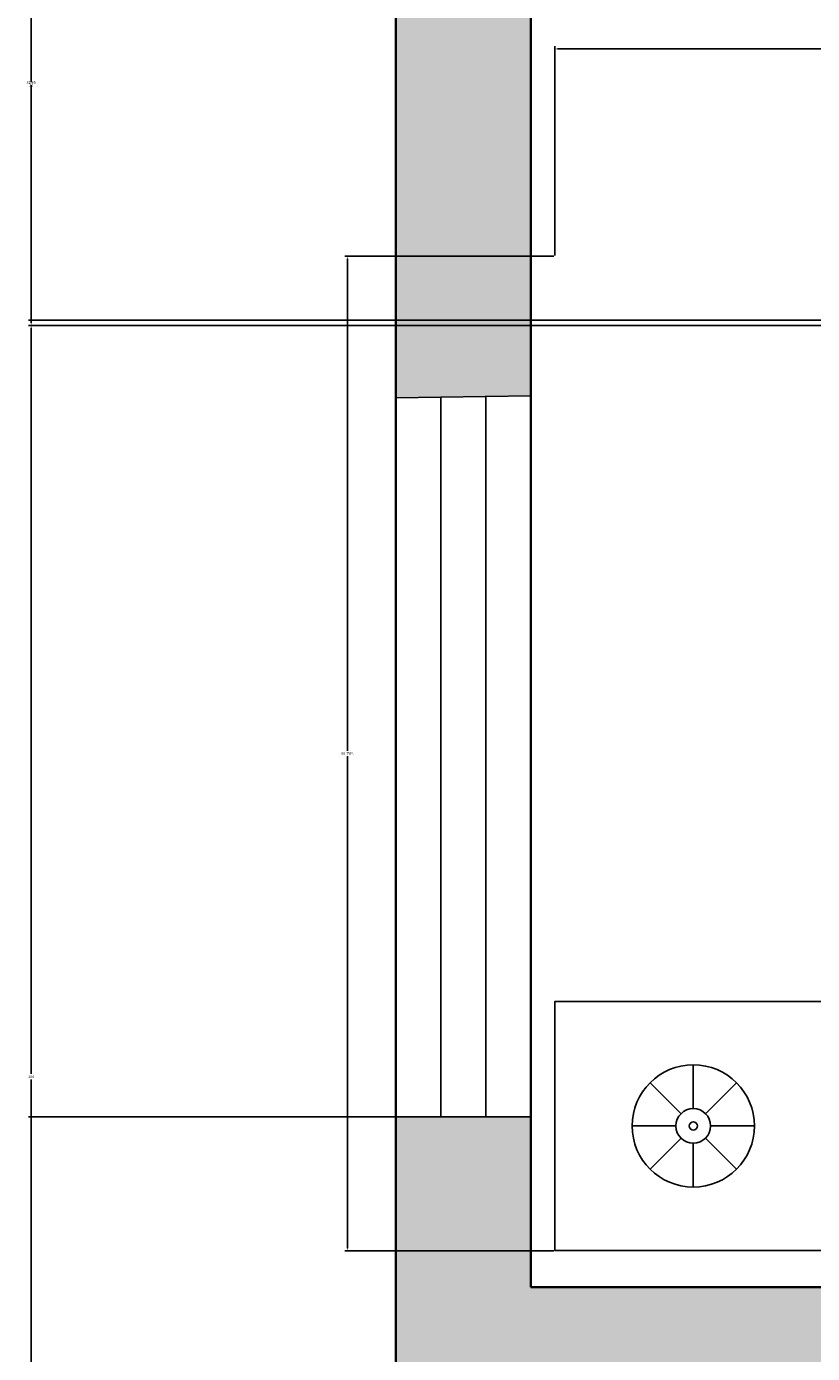
# Model space of a CAD drawing. Units: millimetres. Extents: x 2817 to 5038, y 1110 to 3565.
# Tile 11 of 21: x 2817 to 2869, y 1505 to 1593. Entities that reach past the tile are written whole.
import ezdxf

# ---------------------------------------------------------------- set-up
doc = ezdxf.new("R2010")
doc.units = ezdxf.units.MM
for name, color, linetype, lineweight in [('A-ANNO-DIMS', 2, 'Continuous', 18), ('A-WALL', 7, 'Continuous', 35), ('DOOR&WINDOW', 1, 'Continuous', 25), ('FURNITURE', 219, 'Continuous', 18)]:
    doc.layers.add(name, color=color, linetype=linetype, lineweight=lineweight)
doc.layers.add('A-WALL-PATT', color=51, linetype='Continuous', lineweight=13, true_color=0xf7f281)
doc.layers.add('BLOCK', color=6, linetype='Continuous')
doc.styles.get("Standard").update_dxf_attribs({"font": 'arial.ttf'})
doc.dimstyles.get("Standard").update_dxf_attribs({"dimtxt": 0.18, "dimasz": 0.18, "dimexe": 0.18, "dimexo": 0.0625, "dimgap": 0.09, "dimtad": 0, "dimtih": 1, "dimtoh": 1, "dimdec": 4, "dimzin": 0, "dimdsep": 46, "dimtxsty": 'Standard', "dimcen": 0.09, "dimadec": 0, "dimazin": 0, "dimtfac": 1, "dimtdec": 4, "dimtofl": 0, "dimtmove": 0, "dimatfit": 3, "dimfxl": 1, "dimtolj": 1, "dimtzin": 0, "dimarcsym": 0})

# ---------------------------------------------------------------- blocks, each defined once
blk = doc.blocks.new('A$C52E67D0D')
at = {"layer": 'BLOCK'}
for p, q in [((2251.5, 1605.5), (2251.5, 1684.7)), ((2229.3, 1596.3), (2173.3, 1652.3)), ((2273.7, 1596.3), (2329.7, 1652.3)), ((2220.1, 1574.1), (2140.9, 1574.1)), ((2282.9, 1574.1), (2362.1, 1574.1)), ((2229.3, 1551.9), (2173.3, 1495.9)), ((2251.5, 1542.8), (2251.5, 1463.5)), ((2273.7, 1551.9), (2329.7, 1495.9))]:
    blk.add_line(p, q, dxfattribs=at)
blk.add_lwpolyline([(2001, 1348.6), (2001, 1799.6), (2502, 1799.6), (2502, 1348.6)], close=True, dxfattribs=at)
for radius in [110.6, 31.4, 7.46]:
    blk.add_circle((2251.5, 1574.1), radius, dxfattribs=at)
blk = doc.blocks.new('WIN-4FT')
for p, q in [((0, 0), (0.001, 47.853)), ((0.001, 47.853), (9, 48)), ((3, 0), (3.001, 47.853)), ((6, 48), (6, 0)), ((9, 48), (9, 0)), ((9, 0), (0, 0))]:
    blk.add_line(p, q)
blk = doc.blocks.new('*D18')
at = {"layer": 'A-ANNO-DIMS', "color": 0, "lineweight": -2, "transparency": 16777216}
for p, q in [((2852.329, 1578.101), (2852.329, 1592.019)), ((2852.509, 1591.839), (2897.232, 1591.839)), ((2944.149, 1591.839), (2899.426, 1591.839)), ((2944.329, 1578.101), (2944.329, 1592.019))]:
    blk.add_line(p, q, dxfattribs=at)
for points in [[(2852.509, 1591.869), (2852.509, 1591.809), (2852.329, 1591.839)], [(2944.149, 1591.869), (2944.149, 1591.809), (2944.329, 1591.839)]]:
    blk.add_solid(points, dxfattribs=at)
at = {"layer": 'Defpoints', "color": 0, "lineweight": -2, "transparency": 16777216}
for p in [(2852.329, 1591.839), (2852.329, 1578.039), (2944.329, 1578.039)]:
    blk.add_point(p, dxfattribs=at)
at = {"layer": 'A-ANNO-DIMS', "color": 0, "transparency": 16777216, "insert": (2898.329, 1591.839), "char_height": 0.18, "attachment_point": 5}
blk.add_mtext('\\A1;BED SET 92 TYP.', dxfattribs=at)
blk = doc.blocks.new('*D19')
at = {"layer": 'A-ANNO-DIMS', "color": 0, "lineweight": -2, "transparency": 16777216}
for p, q in [((2852.266, 1578.039), (2838.349, 1578.039)), ((2838.529, 1577.859), (2838.529, 1545.127)), ((2838.529, 1512.031), (2838.529, 1544.763)), ((2852.266, 1511.851), (2838.349, 1511.851))]:
    blk.add_line(p, q, dxfattribs=at)
for points in [[(2838.499, 1577.859), (2838.559, 1577.859), (2838.529, 1578.039)], [(2838.499, 1512.031), (2838.559, 1512.031), (2838.529, 1511.851)]]:
    blk.add_solid(points, dxfattribs=at)
at = {"layer": 'Defpoints', "color": 0, "lineweight": -2, "transparency": 16777216}
for p in [(2852.329, 1578.039), (2838.529, 1511.851), (2852.329, 1511.851)]:
    blk.add_point(p, dxfattribs=at)
at = {"layer": 'A-ANNO-DIMS', "color": 0, "transparency": 16777216, "insert": (2838.529, 1544.945), "char_height": 0.18, "attachment_point": 5}
blk.add_mtext('\\A1;66 TYP.', dxfattribs=at)
blk = doc.blocks.new('*D33')
at = {"layer": 'A-ANNO-DIMS', "color": 0, "lineweight": -2, "transparency": 16777216}
for p, q in [((2841.676, 1520.761), (2817.308, 1520.761)), ((2817.488, 1520.581), (2817.488, 1474.171)), ((2817.488, 1427.398), (2817.488, 1473.807)), ((2841.677, 1427.218), (2817.308, 1427.218))]:
    blk.add_line(p, q, dxfattribs=at)
for points in [[(2817.458, 1520.581), (2817.518, 1520.581), (2817.488, 1520.761)], [(2817.458, 1427.398), (2817.518, 1427.398), (2817.488, 1427.218)]]:
    blk.add_solid(points, dxfattribs=at)
at = {"layer": 'Defpoints', "color": 0, "lineweight": -2, "transparency": 16777216}
for p in [(2817.488, 1520.761), (2841.738, 1520.761), (2841.739, 1427.218)]:
    blk.add_point(p, dxfattribs=at)
at = {"layer": 'A-ANNO-DIMS', "color": 0, "transparency": 16777216, "insert": (2817.488, 1473.989), "char_height": 0.18, "attachment_point": 5}
blk.add_mtext('\\A1;93.54', dxfattribs=at)
blk = doc.blocks.new('*D38')
at = {"layer": 'A-ANNO-DIMS', "color": 0, "lineweight": -2, "transparency": 16777216}
for p, q in [((3110.177, 1573.436), (2817.308, 1573.436)), ((2817.488, 1573.256), (2817.488, 1523.618)), ((2817.488, 1473.616), (2817.488, 1523.254)), ((3105.677, 1473.436), (2817.308, 1473.436))]:
    blk.add_line(p, q, dxfattribs=at)
for points in [[(2817.458, 1573.256), (2817.518, 1573.256), (2817.488, 1573.436)], [(2817.458, 1473.616), (2817.518, 1473.616), (2817.488, 1473.436)]]:
    blk.add_solid(points, dxfattribs=at)
at = {"layer": 'Defpoints', "color": 0, "lineweight": -2, "transparency": 16777216}
for p in [(2817.488, 1573.436), (3110.239, 1573.436), (3105.739, 1473.436)]:
    blk.add_point(p, dxfattribs=at)
at = {"layer": 'A-ANNO-DIMS', "color": 0, "transparency": 16777216, "insert": (2817.488, 1523.436), "char_height": 0.18, "attachment_point": 5}
blk.add_mtext('\\A1;100', dxfattribs=at)
blk = doc.blocks.new('*D39')
at = {"layer": 'A-ANNO-DIMS', "color": 0, "lineweight": -2, "transparency": 16777216}
for p, q in [((3105.677, 1605.436), (2817.308, 1605.436)), ((2817.488, 1605.256), (2817.488, 1589.618)), ((2817.488, 1573.616), (2817.488, 1589.254)), ((3110.177, 1573.436), (2817.308, 1573.436))]:
    blk.add_line(p, q, dxfattribs=at)
for points in [[(2817.458, 1605.256), (2817.518, 1605.256), (2817.488, 1605.436)], [(2817.458, 1573.616), (2817.518, 1573.616), (2817.488, 1573.436)]]:
    blk.add_solid(points, dxfattribs=at)
at = {"layer": 'Defpoints', "color": 0, "lineweight": -2, "transparency": 16777216}
for p in [(2817.488, 1605.436), (3105.739, 1605.436), (3110.239, 1573.436)]:
    blk.add_point(p, dxfattribs=at)
at = {"layer": 'A-ANNO-DIMS', "color": 0, "transparency": 16777216, "insert": (2817.488, 1589.436), "char_height": 0.18, "attachment_point": 5}
blk.add_mtext('\\A1;32', dxfattribs=at)
blk = doc.blocks.new('*D46')
at = {"layer": 'A-ANNO-DIMS', "color": 0, "lineweight": -2, "transparency": 16777216}
for p, q in [((3052.177, 1605.436), (2817.308, 1605.436)), ((2817.488, 1605.256), (2817.488, 1589.792)), ((2817.488, 1573.964), (2817.488, 1589.428)), ((3052.075, 1573.784), (2817.308, 1573.784))]:
    blk.add_line(p, q, dxfattribs=at)
for points in [[(2817.458, 1605.256), (2817.518, 1605.256), (2817.488, 1605.436)], [(2817.458, 1573.964), (2817.518, 1573.964), (2817.488, 1573.784)]]:
    blk.add_solid(points, dxfattribs=at)
at = {"layer": 'Defpoints', "color": 0, "lineweight": -2, "transparency": 16777216}
for p in [(2817.488, 1605.436), (3052.239, 1605.436), (3052.138, 1573.784)]:
    blk.add_point(p, dxfattribs=at)
at = {"layer": 'A-ANNO-DIMS', "color": 0, "transparency": 16777216, "insert": (2817.488, 1589.61), "char_height": 0.18, "attachment_point": 5}
blk.add_mtext('\\A1;31.65', dxfattribs=at)

msp = doc.modelspace()

# ---------------------------------------------------------------- hatches: boundary and pattern name
at = {"layer": 'A-WALL-PATT'}
h = msp.add_hatch(color=256, dxfattribs=at)
h.dxf.hatch_style = 1
h.paths.add_polyline_path([(3186.7393, 1614.4357), (2841.7393, 1614.4357), (2841.7393, 1568.614), (2850.7393, 1568.7609), (2850.7393, 1605.4357), (2982.7393, 1605.4357), (2991.7393, 1605.4357), (3052.2393, 1605.4357), (3052.2393, 1573.7835), (3061.2393, 1573.7835), (3061.2393, 1605.4357), (3182.2393, 1605.4357), (3182.2393, 1143.4357), (3181.2393, 1143.4357), (3181.2393, 1134.4357), (3186.7393, 1134.4357)])
h.paths.add_polyline_path([(3061.2393, 1143.4357), (3061.2393, 1147.4357), (3052.2393, 1147.4357), (3052.2393, 1143.4357), (2850.7393, 1143.4357), (2850.7393, 1145.2996), (2841.7393, 1145.2996), (2841.7393, 1134.4357), (3061.2393, 1134.4357)], flags=17)
h.paths.add_polyline_path([(2850.7393, 1265.4357), (2946.7393, 1265.4357), (2946.7393, 1270.8357), (2946.7393, 1274.4357), (2850.7393, 1274.4357), (2850.7381, 1274.4357), (2850.7381, 1274.2564), (2841.7393, 1274.2564), (2841.7393, 1193.1527), (2850.7393, 1193.2996)], flags=17)
h.paths.add_polyline_path([(3061.2393, 1299.098), (3052.2393, 1299.098), (3052.2393, 1274.4357), (2991.7393, 1274.4357), (2991.7393, 1340.4357), (2982.7393, 1340.4357), (2982.7393, 1274.4357), (2982.7393, 1265.4357), (3052.2393, 1265.4357), (3052.2393, 1259.143), (3061.2393, 1259.2899)], flags=17)
h.paths.add_polyline_path([(3061.2393, 1383.4357), (3052.2393, 1383.4357), (3052.2393, 1379.4357), (2931.7393, 1379.4357), (2922.7393, 1379.4357), (2850.7393, 1379.4357), (2850.7381, 1379.4357), (2850.7381, 1379.3646), (2841.7393, 1379.3646), (2841.7393, 1322.1095), (2850.7393, 1322.2564), (2850.7393, 1370.4357), (2982.7393, 1370.4357), (2987.2393, 1370.4357), (3017.2393, 1370.4357), (3052.2393, 1370.4357), (3052.2393, 1323.098), (3061.2393, 1323.098)], flags=17)
h = msp.add_hatch(color=256, dxfattribs=at)
h.dxf.hatch_style = 1
h.paths.add_polyline_path([(3061.2393, 1549.7835), (3052.2393, 1549.7835), (3052.2393, 1509.4357), (2991.7393, 1509.4357), (2991.7393, 1575.4357), (2982.7393, 1575.4357), (2982.7393, 1509.4357), (2982.7393, 1500.4357), (3052.2393, 1500.4357), (3052.2393, 1498.4661), (3061.2393, 1498.613)])
h.paths.add_polyline_path([(2946.7393, 1505.8357), (2946.7393, 1509.4357), (2850.7393, 1509.4357), (2850.7393, 1520.7609), (2841.7393, 1520.7609), (2841.7393, 1427.2177), (2850.7393, 1427.3646), (2850.7393, 1500.4357), (2922.7393, 1500.4357), (2931.7393, 1500.4357), (2946.7393, 1500.4357)])
h.paths.add_polyline_path([(3061.2393, 1450.613), (3052.2393, 1450.613), (3052.2393, 1431.4357), (3059.4393, 1431.4357), (3061.2393, 1431.4357)])
h.paths.add_polyline_path([(3061.2393, 1211.2899), (3052.2393, 1211.2899), (3052.2393, 1195.4357), (3059.4393, 1195.4357), (3061.2393, 1195.4357)])

# ---------------------------------------------------------------- linework, layer by layer
at = {"layer": 'A-WALL'}
for p, q in [((2841.7393, 1134.4357), (2841.7393, 1614.4357)), ((2850.7393, 1509.4357), (2850.7393, 1605.4357)), ((2850.7393, 1509.4357), (2946.7393, 1509.4357))]:
    msp.add_line(p, q, dxfattribs=at)

# ---------------------------------------------------------------- block references
at = {"layer": 'DOOR&WINDOW'}
msp.add_blockref('WIN-4FT', (2841.7381, 1520.7608), dxfattribs=at)
at = {"layer": 'FURNITURE', "xscale": 0.0367705835331598, "yscale": 0.0367705835331598, "zscale": 0.0367705835331598, "rotation": 180}
msp.add_blockref('A$C52E67D0D', (2944.3285, 1578.0385), dxfattribs=at)

# ---------------------------------------------------------------- dimensions: what is measured, and where the dimension line sits
at = {"layer": 'A-ANNO-DIMS'}
for base, p1, p2, override, picture, middle in [((2817.4881, 1605.4357), (3052.1378, 1573.7835), (3052.2393, 1605.4357), {"dimdec": 2, "dimlfac": 1, "dimrnd": 0, "dimzin": 0, "dimdsep": 46, "dimlunit": 2}, '*D46', (2817.4881, 1589.6096)), ((2817.4881, 1605.4357), (3110.2393, 1573.4357), (3105.7393, 1605.4357), {"dimdec": 0, "dimlfac": 1, "dimrnd": 0, "dimzin": 0, "dimdsep": 46, "dimlunit": 2}, '*D39', (2817.4881, 1589.4357)), ((2817.4881, 1573.4357), (3105.7393, 1473.4357), (3110.2393, 1573.4357), {"dimdec": 0, "dimlfac": 1, "dimrnd": 0, "dimzin": 0, "dimdsep": 46, "dimlunit": 2}, '*D38', (2817.4881, 1523.4357)), ((2817.4881, 1520.7609), (2841.7393, 1427.2177), (2841.7381, 1520.7609), {"dimdec": 2, "dimlfac": 1, "dimrnd": 0, "dimzin": 0, "dimdsep": 46, "dimlunit": 2}, '*D33', (2817.4881, 1473.9893))]:
    dim = msp.add_linear_dim(base=base, p1=p1, p2=p2, angle=90, dimstyle='Standard', override=override, dxfattribs=at)
    dim.commit()
    dim.dimension.update_dxf_attribs({"geometry": picture, "text_midpoint": middle})
for base, p1, p2, angle, text, picture, middle in [((2852.3285, 1591.8385), (2944.3285, 1578.0385), (2852.3285, 1578.0385), 180, 'BED SET <> TYP.', '*D18', (2898.3285, 1591.8385)), ((2838.5285, 1511.8515), (2852.3285, 1578.0385), (2852.3285, 1511.8515), 270, '<> TYP.', '*D19', (2838.5285, 1544.945))]:
    dim = msp.add_linear_dim(base=base, p1=p1, p2=p2, angle=angle, text=text, dimstyle='Standard', override={"dimdec": 0, "dimlfac": 1, "dimrnd": 0, "dimzin": 0, "dimdsep": 46, "dimlunit": 2}, dxfattribs=at)
    dim.commit()
    dim.dimension.update_dxf_attribs({"geometry": picture, "text_midpoint": middle})

doc.saveas('drawing.dxf')
